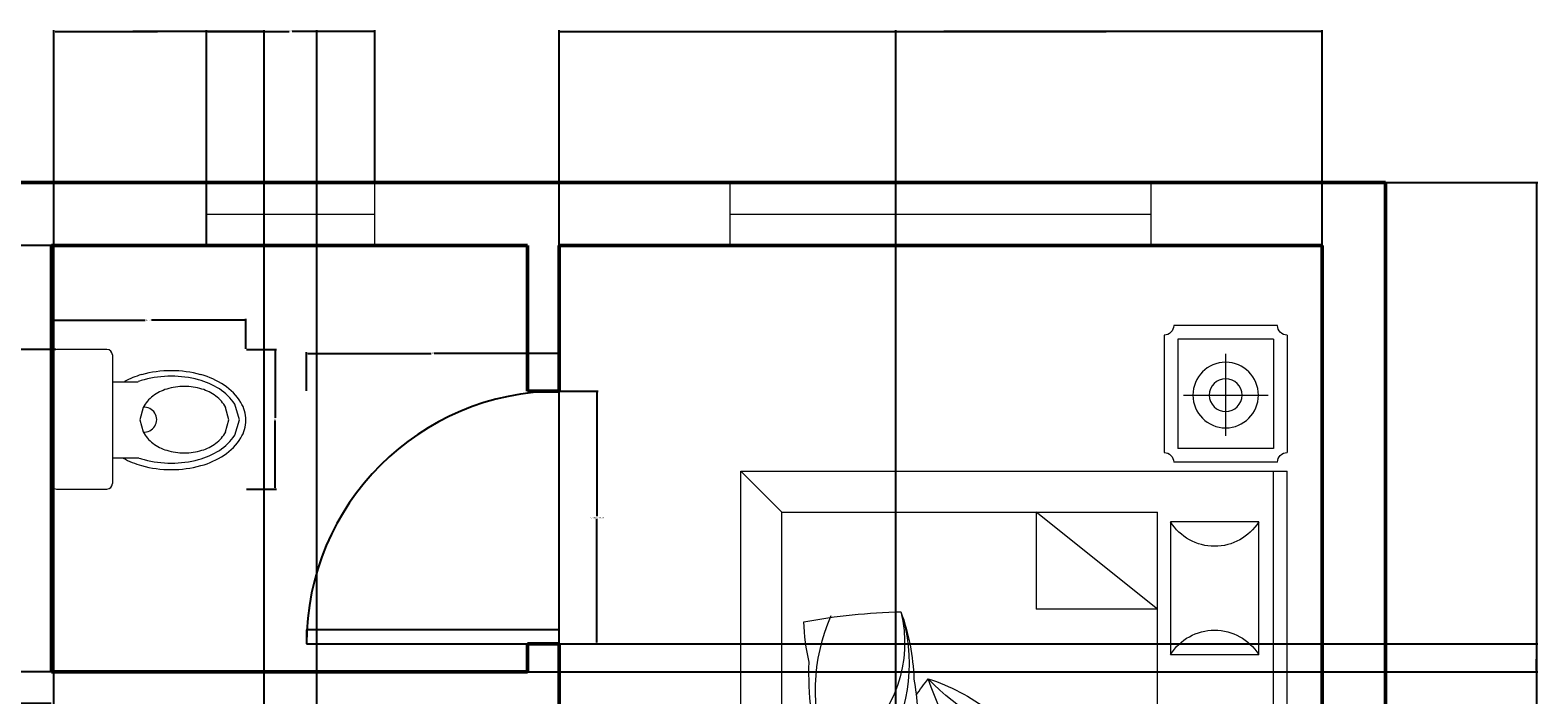
# Model space of a CAD drawing. Units: inches. Extents: x -108 to 1456, y -102 to 617.
# Tile 7 of 8: x 345 to 560, y 523 to 617. Entities that reach past the tile are written whole.
import ezdxf

# ---------------------------------------------------------------- set-up
doc = ezdxf.new("R2010")
doc.units = ezdxf.units.IN
for name, color, linetype, lineweight in [('A-ANNO-DIMS', 2, 'Continuous', 18), ('A-DOOR', 3, 'Continuous', 25), ('A-FLOR-FIXT', 9, 'Continuous', 20), ('A-FURN', 8, 'Continuous', 18), ('A-GLAZ', 4, 'Continuous', 18), ('A-WALL', 7, 'Continuous', 50)]:
    doc.layers.add(name, color=color, linetype=linetype, lineweight=lineweight)
doc.styles.get("Standard").update_dxf_attribs({"font": 'arial.ttf'})
doc.dimstyles.get("Standard").update_dxf_attribs({"dimtxt": 0.18, "dimasz": 0.18, "dimexe": 0.18, "dimexo": 0.0625, "dimgap": 0.09, "dimtad": 0, "dimtih": 1, "dimtoh": 1, "dimdec": 4, "dimzin": 0, "dimdsep": 46, "dimtxsty": 'Standard', "dimcen": 0.09, "dimadec": 0, "dimazin": 0, "dimtfac": 1, "dimtdec": 4, "dimtofl": 0, "dimtmove": 0, "dimatfit": 3, "dimfxl": 1, "dimtolj": 1, "dimtzin": 0, "dimarcsym": 0})

# ---------------------------------------------------------------- blocks, each defined once
blk = doc.blocks.new('A$C50B66110')
for p, q in [((0.0503, 1.9981), (0.4803, 1.9981)), ((0.1513, 1.6871), (0.1513, 1.9967)), ((0.5716, 1.9488), (0.5716, 2)), ((0.5716, 2), (2.0719, 2)), ((2.0719, 1.9488), (2.0719, 2)), ((2.5701, 1.9993), (2.1401, 1.9993)), ((0.0153, 1.9631), (0.0153, 1.5831)), ((0.0653, 1.9481), (0.0653, 1.5981)), ((0.0653, 1.9481), (0.4653, 1.9481)), ((0.4653, 1.9481), (0.4653, 1.5981)), ((0.5153, 1.9631), (0.5153, 1.5831)), ((2.0719, 1.9488), (0.5716, 1.9488)), ((0.5716, 1.9488), (0.5716, 0)), ((2.0719, 0), (2.0719, 1.9488)), ((2.1051, 1.9643), (2.1051, 1.5843)), ((2.1551, 1.9493), (2.1551, 1.5993)), ((2.5551, 1.9493), (2.1551, 1.9493)), ((2.5551, 1.9493), (2.5551, 1.5993)), ((2.6051, 1.9643), (2.6051, 1.5843)), ((0.7257, 1.5725), (0.7257, 1.8954)), ((0.7257, 1.8954), (1.2113, 1.8954)), ((1.2113, 1.8954), (1.2113, 1.5725)), ((1.4007, 1.5725), (1.4007, 1.8954)), ((1.4007, 1.8954), (1.8863, 1.8954)), ((1.8863, 1.8954), (1.8863, 1.5725)), ((2.3505, 1.62), (2.3505, 1.9295)), ((0, 1.8416), (0.2001, 1.8416)), ((2.5018, 1.7744), (2.2017, 1.7744)), ((0.0503, 1.5481), (0.4803, 1.5481)), ((0.0653, 1.5981), (0.4653, 1.5981)), ((1.2113, 1.5725), (0.7257, 1.5725)), ((1.8863, 1.5725), (1.4007, 1.5725)), ((2.5701, 1.5493), (2.1401, 1.5493)), ((2.5551, 1.5993), (2.1551, 1.5993)), ((1.5665, 1.5254), (1.5665, 1.0802)), ((1.5665, 1.5254), (1.9219, 1.0802)), ((1.9219, 1.0802), (1.5665, 1.0802)), ((0.5716, 0), (0.7216, 0.15)), ((2.0719, 0), (1.9219, 0.15)), ((0.5716, 0), (2.0719, 0))]:
    blk.add_line(p, q)
at = {"linetype": 'ByBlock'}
for p, q in [((0.2481, 1.9162), (0.2458, 1.9139)), ((0.2458, 1.9139), (0.2458, 1.7562)), ((0.2481, 1.9162), (0.4287, 1.9162)), ((0.2526, 1.9036), (0.2526, 1.8431)), ((0.3669, 1.9036), (0.2526, 1.9036)), ((0.3669, 1.8431), (0.3669, 1.9036)), ((0.3772, 1.9071), (0.3818, 1.9128)), ((0.3772, 1.7688), (0.3772, 1.9071)), ((0.3818, 1.9094), (0.3807, 1.9048)), ((0.3807, 1.9048), (0.3807, 1.8739)), ((0.3807, 1.9048), (0.3909, 1.8945)), ((0.3818, 1.9128), (0.4161, 1.9128)), ((0.3864, 1.9116), (0.3818, 1.9094)), ((0.3921, 1.8968), (0.3864, 1.9116)), ((0.3864, 1.9116), (0.4138, 1.9116)), ((0.3909, 1.8945), (0.3921, 1.8968)), ((0.3909, 1.8431), (0.3909, 1.8945)), ((0.4081, 1.8968), (0.3921, 1.8968)), ((0.4081, 1.8968), (0.4138, 1.9116)), ((0.4092, 1.8945), (0.4081, 1.8968)), ((0.4195, 1.9048), (0.4092, 1.8945)), ((0.4092, 1.8431), (0.4092, 1.8945)), ((0.4138, 1.9116), (0.4184, 1.9094)), ((0.4161, 1.9128), (0.4218, 1.9071)), ((0.4184, 1.9094), (0.4195, 1.9048)), ((0.4195, 1.9048), (0.4195, 1.8739)), ((0.4218, 1.9071), (0.4218, 1.7699)), ((0.4287, 1.9162), (0.4309, 1.9139)), ((0.4309, 1.9139), (0.4309, 1.7562)), ((0.2526, 1.8431), (0.3669, 1.8431)), ((0.2572, 1.8408), (0.2572, 1.8294)), ((0.3669, 1.8408), (0.2572, 1.8408)), ((0.2572, 1.8294), (0.3669, 1.8294)), ((0.2664, 1.8408), (0.2664, 1.8294)), ((0.2755, 1.8408), (0.2755, 1.8294)), ((0.2846, 1.8408), (0.2846, 1.8294)), ((0.2938, 1.8408), (0.2938, 1.8294)), ((0.3029, 1.8408), (0.3029, 1.8294)), ((0.3121, 1.8408), (0.3121, 1.8294)), ((0.3669, 1.8294), (0.3669, 1.8408)), ((0.3807, 1.8739), (0.3829, 1.8682)), ((0.3829, 1.8682), (0.3864, 1.8625)), ((0.3864, 1.8625), (0.3875, 1.8545)), ((0.3864, 1.8134), (0.3875, 1.8214)), ((0.3875, 1.8545), (0.3875, 1.8431)), ((0.3875, 1.8214), (0.3875, 1.8431)), ((0.3909, 1.8431), (0.3909, 1.7813)), ((0.4092, 1.8431), (0.4092, 1.7813)), ((0.4138, 1.8625), (0.4127, 1.8545)), ((0.4127, 1.8545), (0.4127, 1.8431)), ((0.4127, 1.8214), (0.4127, 1.8431)), ((0.4138, 1.8134), (0.4127, 1.8214)), ((0.4172, 1.8682), (0.4138, 1.8625)), ((0.4195, 1.8739), (0.4172, 1.8682)), ((0.3201, 1.8168), (0.2526, 1.8168)), ((0.2526, 1.8168), (0.2526, 1.7962)), ((0.2526, 1.7962), (0.3201, 1.7962)), ((0.2652, 1.7905), (0.2538, 1.7905)), ((0.2538, 1.7905), (0.2538, 1.7859)), ((0.2538, 1.7859), (0.2652, 1.7859)), ((0.2538, 1.7665), (0.2538, 1.7733)), ((0.2538, 1.7733), (0.2652, 1.7733)), ((0.2652, 1.7665), (0.2538, 1.7665)), ((0.2675, 1.8145), (0.2641, 1.8145)), ((0.2641, 1.8145), (0.2641, 1.8111)), ((0.2641, 1.8111), (0.2675, 1.8111)), ((0.2641, 1.8019), (0.2641, 1.7985)), ((0.2675, 1.8019), (0.2641, 1.8019)), ((0.2641, 1.7985), (0.2675, 1.7985)), ((0.2652, 1.7859), (0.2652, 1.7905)), ((0.2652, 1.7733), (0.2652, 1.7665)), ((0.2675, 1.8111), (0.2675, 1.8145)), ((0.2675, 1.7985), (0.2675, 1.8019)), ((0.2812, 1.7905), (0.2698, 1.7905)), ((0.2698, 1.7905), (0.2698, 1.7859)), ((0.2698, 1.7859), (0.2812, 1.7859)), ((0.2698, 1.7665), (0.2698, 1.7733)), ((0.2698, 1.7733), (0.2812, 1.7733)), ((0.2812, 1.7665), (0.2698, 1.7665)), ((0.2812, 1.7859), (0.2812, 1.7905)), ((0.2812, 1.7733), (0.2812, 1.7665)), ((0.2846, 1.8145), (0.2846, 1.8111)), ((0.2881, 1.8145), (0.2846, 1.8145)), ((0.2846, 1.8111), (0.2881, 1.8111)), ((0.2846, 1.8019), (0.2846, 1.7985)), ((0.2881, 1.8019), (0.2846, 1.8019)), ((0.2846, 1.7985), (0.2881, 1.7985)), ((0.2972, 1.7905), (0.2858, 1.7905)), ((0.2858, 1.7905), (0.2858, 1.7859)), ((0.2858, 1.7859), (0.2972, 1.7859)), ((0.2858, 1.7665), (0.2858, 1.7733)), ((0.2858, 1.7733), (0.2972, 1.7733)), ((0.2972, 1.7665), (0.2858, 1.7665)), ((0.2881, 1.8111), (0.2881, 1.8145)), ((0.2881, 1.7985), (0.2881, 1.8019)), ((0.2972, 1.7859), (0.2972, 1.7905)), ((0.2972, 1.7733), (0.2972, 1.7665)), ((0.3018, 1.7905), (0.3018, 1.7859)), ((0.3132, 1.7905), (0.3018, 1.7905)), ((0.3018, 1.7859), (0.3132, 1.7859)), ((0.3018, 1.7733), (0.3132, 1.7733)), ((0.3018, 1.7665), (0.3018, 1.7733)), ((0.3132, 1.7665), (0.3018, 1.7665)), ((0.3052, 1.8145), (0.3052, 1.8111)), ((0.3086, 1.8145), (0.3052, 1.8145)), ((0.3052, 1.8111), (0.3086, 1.8111)), ((0.3052, 1.8019), (0.3052, 1.7985)), ((0.3086, 1.8019), (0.3052, 1.8019)), ((0.3052, 1.7985), (0.3086, 1.7985)), ((0.3086, 1.8111), (0.3086, 1.8145)), ((0.3086, 1.7985), (0.3086, 1.8019)), ((0.3132, 1.7859), (0.3132, 1.7905)), ((0.3132, 1.7733), (0.3132, 1.7665)), ((0.3201, 1.7962), (0.3201, 1.8168)), ((0.3304, 1.8111), (0.3395, 1.8111)), ((0.3304, 1.8042), (0.3304, 1.8111)), ((0.3395, 1.8042), (0.3304, 1.8042)), ((0.3304, 1.7985), (0.3395, 1.7985)), ((0.3304, 1.7916), (0.3304, 1.7985)), ((0.3395, 1.7916), (0.3304, 1.7916)), ((0.3304, 1.7779), (0.3304, 1.7848)), ((0.3304, 1.7848), (0.3395, 1.7848)), ((0.3395, 1.7779), (0.3304, 1.7779)), ((0.3304, 1.7722), (0.3395, 1.7722)), ((0.3304, 1.7653), (0.3304, 1.7722)), ((0.3395, 1.8111), (0.3395, 1.8042)), ((0.3395, 1.7985), (0.3395, 1.7916)), ((0.3395, 1.7848), (0.3395, 1.7779)), ((0.3395, 1.7722), (0.3395, 1.7653)), ((0.3441, 1.8042), (0.3441, 1.8111)), ((0.3441, 1.8111), (0.3532, 1.8111)), ((0.3532, 1.8042), (0.3441, 1.8042)), ((0.3441, 1.7985), (0.3532, 1.7985)), ((0.3441, 1.7916), (0.3441, 1.7985)), ((0.3532, 1.7916), (0.3441, 1.7916)), ((0.3441, 1.7779), (0.3441, 1.7848)), ((0.3441, 1.7848), (0.3532, 1.7848)), ((0.3532, 1.7779), (0.3441, 1.7779)), ((0.3441, 1.7722), (0.3532, 1.7722)), ((0.3441, 1.7653), (0.3441, 1.7722)), ((0.3532, 1.8111), (0.3532, 1.8042)), ((0.3532, 1.7985), (0.3532, 1.7916)), ((0.3532, 1.7848), (0.3532, 1.7779)), ((0.3532, 1.7722), (0.3532, 1.7653)), ((0.3578, 1.8111), (0.3669, 1.8111)), ((0.3578, 1.8042), (0.3578, 1.8111)), ((0.3669, 1.8042), (0.3578, 1.8042)), ((0.3578, 1.7985), (0.3669, 1.7985)), ((0.3578, 1.7916), (0.3578, 1.7985)), ((0.3669, 1.7916), (0.3578, 1.7916)), ((0.3578, 1.7791), (0.3578, 1.7859)), ((0.3578, 1.7859), (0.3669, 1.7859)), ((0.3669, 1.7791), (0.3578, 1.7791)), ((0.3578, 1.7653), (0.3578, 1.7722)), ((0.3578, 1.7722), (0.3669, 1.7722)), ((0.3669, 1.8111), (0.3669, 1.8042)), ((0.3669, 1.7985), (0.3669, 1.7916)), ((0.3669, 1.7859), (0.3669, 1.7791)), ((0.3669, 1.7722), (0.3669, 1.7653)), ((0.3829, 1.7631), (0.3772, 1.7688)), ((0.3807, 1.8019), (0.3829, 1.8076)), ((0.3807, 1.7711), (0.3807, 1.8019)), ((0.3807, 1.7711), (0.3909, 1.7813)), ((0.3818, 1.7665), (0.3807, 1.7711)), ((0.3864, 1.7642), (0.3818, 1.7665)), ((0.3829, 1.8076), (0.3864, 1.8134)), ((0.3921, 1.7791), (0.3864, 1.7642)), ((0.3909, 1.7813), (0.3921, 1.7791)), ((0.4081, 1.7791), (0.3921, 1.7791)), ((0.4024, 1.7676), (0.3989, 1.7676)), ((0.3989, 1.7676), (0.3991, 1.7578)), ((0.403, 1.7585), (0.4024, 1.7676)), ((0.4092, 1.7813), (0.4081, 1.7791)), ((0.4081, 1.7791), (0.4138, 1.7642)), ((0.4195, 1.7711), (0.4092, 1.7813)), ((0.4172, 1.8076), (0.4138, 1.8134)), ((0.4138, 1.7642), (0.4184, 1.7665)), ((0.4218, 1.7699), (0.4161, 1.7631)), ((0.4195, 1.8019), (0.4172, 1.8076)), ((0.4184, 1.7665), (0.4195, 1.7711)), ((0.4195, 1.7711), (0.4195, 1.8019)), ((0.4378, 1.7742), (0.4309, 1.7768)), ((0.4309, 1.7722), (0.436, 1.7708)), ((0.436, 1.7708), (0.4406, 1.7672)), ((0.441, 1.771), (0.4378, 1.7742)), ((0.4406, 1.7672), (0.4418, 1.7656)), ((0.4434, 1.7688), (0.441, 1.771)), ((0.4477, 1.7704), (0.4434, 1.7688)), ((0.4497, 1.7684), (0.4477, 1.7704)), ((0.4481, 1.765), (0.4497, 1.7684)), ((0.4509, 1.7672), (0.4481, 1.765)), ((0.4539, 1.764), (0.4509, 1.7672)), ((0.2458, 1.7562), (0.2481, 1.7539)), ((0.4, 1.7539), (0.2481, 1.7539)), ((0.3395, 1.7653), (0.3304, 1.7653)), ((0.3532, 1.7653), (0.3441, 1.7653)), ((0.3669, 1.7653), (0.3578, 1.7653)), ((0.399, 1.7631), (0.3829, 1.7631)), ((0.3864, 1.7642), (0.399, 1.7642)), ((0.3991, 1.7578), (0.4019, 1.7462)), ((0.4019, 1.7462), (0.4047, 1.7353)), ((0.4026, 1.7254), (0.4021, 1.7198)), ((0.4021, 1.7198), (0.4088, 1.7187)), ((0.4088, 1.7187), (0.4023, 1.7147)), ((0.4023, 1.7147), (0.4028, 1.7085)), ((0.4026, 1.7642), (0.4138, 1.7642)), ((0.4051, 1.7279), (0.4026, 1.7254)), ((0.4161, 1.7631), (0.4027, 1.7631)), ((0.4047, 1.7511), (0.403, 1.7585)), ((0.4287, 1.7539), (0.404, 1.7539)), ((0.4047, 1.7353), (0.4044, 1.7293)), ((0.4044, 1.7293), (0.4051, 1.7279)), ((0.4074, 1.7402), (0.4047, 1.7511)), ((0.4081, 1.7346), (0.4074, 1.7402)), ((0.4079, 1.7286), (0.4081, 1.7346)), ((0.4121, 1.7256), (0.4079, 1.7286)), ((0.4111, 1.7203), (0.4121, 1.7256)), ((0.4123, 1.7057), (0.4111, 1.7203)), ((0.4309, 1.7562), (0.4287, 1.7539)), ((0.4443, 1.7658), (0.4418, 1.7633)), ((0.4418, 1.7656), (0.4443, 1.7658)), ((0.4418, 1.7633), (0.4511, 1.7551)), ((0.4511, 1.7551), (0.4662, 1.7422)), ((0.4515, 1.7573), (0.4539, 1.764)), ((0.4577, 1.7605), (0.4515, 1.7573)), ((0.463, 1.7555), (0.4577, 1.7605)), ((0.4618, 1.7482), (0.463, 1.7555)), ((0.467, 1.7515), (0.4618, 1.7482)), ((0.4664, 1.7418), (0.4741, 1.72)), ((0.4714, 1.7468), (0.467, 1.7515)), ((0.4696, 1.7418), (0.4714, 1.7468)), ((0.4766, 1.7425), (0.4697, 1.7418)), ((0.4741, 1.72), (0.4708, 1.7027)), ((0.472, 1.733), (0.4787, 1.7356)), ((0.4794, 1.7332), (0.472, 1.733)), ((0.4761, 1.7233), (0.481, 1.7279)), ((0.4824, 1.7233), (0.4761, 1.7233)), ((0.4764, 1.7154), (0.4835, 1.7175)), ((0.4824, 1.7119), (0.4764, 1.7154)), ((0.4787, 1.7356), (0.4766, 1.7425)), ((0.481, 1.7279), (0.4794, 1.7332)), ((0.4815, 1.7073), (0.4824, 1.7119)), ((0.4835, 1.7175), (0.4824, 1.7233)), ((0.4028, 1.7085), (0.4102, 1.7078)), ((0.4102, 1.7078), (0.4037, 1.7027)), ((0.4037, 1.7027), (0.4067, 1.6974)), ((0.4067, 1.6974), (0.4137, 1.6988)), ((0.4137, 1.6988), (0.4104, 1.6923)), ((0.4104, 1.6923), (0.4139, 1.6881)), ((0.4211, 1.6946), (0.4123, 1.7057)), ((0.4139, 1.6881), (0.4192, 1.692)), ((0.4192, 1.692), (0.4183, 1.6858)), ((0.4183, 1.6858), (0.4227, 1.683)), ((0.4333, 1.6881), (0.4211, 1.6946)), ((0.4227, 1.683), (0.4283, 1.6876)), ((0.4283, 1.6876), (0.4276, 1.68)), ((0.4276, 1.68), (0.4324, 1.6786)), ((0.4324, 1.6786), (0.4354, 1.6849)), ((0.4472, 1.6869), (0.4333, 1.6881)), ((0.4354, 1.6849), (0.4382, 1.6786)), ((0.4382, 1.6786), (0.4421, 1.6782)), ((0.4421, 1.6782), (0.4437, 1.6849)), ((0.4437, 1.6849), (0.4463, 1.6775)), ((0.4463, 1.6775), (0.4507, 1.6786)), ((0.4606, 1.6927), (0.4472, 1.6869)), ((0.4507, 1.6786), (0.4509, 1.6849)), ((0.4509, 1.6849), (0.4562, 1.6802)), ((0.4562, 1.6802), (0.4599, 1.6821)), ((0.4592, 1.689), (0.4641, 1.683)), ((0.4599, 1.6821), (0.4592, 1.689)), ((0.4708, 1.7027), (0.4606, 1.6927)), ((0.4641, 1.683), (0.4678, 1.6863)), ((0.465, 1.6925), (0.4715, 1.6897)), ((0.4678, 1.6863), (0.465, 1.6925)), ((0.4745, 1.6925), (0.4713, 1.6988)), ((0.4713, 1.6988), (0.478, 1.6967)), ((0.4715, 1.6897), (0.4745, 1.6925)), ((0.4743, 1.7075), (0.4815, 1.7073)), ((0.4798, 1.7013), (0.4743, 1.7075)), ((0.478, 1.6967), (0.4798, 1.7013)), ((0.7216, 1.5254), (1.9219, 1.5254)), ((0.7216, 1.5254), (0.7216, 0.15)), ((1.9219, 0.15), (1.9219, 1.5254)), ((0.7216, 0.15), (1.9219, 0.15))]:
    blk.add_line(p, q, dxfattribs=at)
for centre, radius in [((0.1513, 1.8416), 0.12), ((0.1513, 1.8416), 0.06), ((2.3505, 1.7744), 0.12), ((2.3505, 1.7744), 0.06)]:
    blk.add_circle(centre, radius)
for centre, radius, start, end in [((0.0153, 1.9981), 0.035, 270, 0), ((0.5153, 1.9981), 0.035, 180, 270), ((2.1051, 1.9993), 0.035, 270, 0), ((2.6051, 1.9993), 0.035, 180, 270), ((0.6244, 1.734), 0.1906, 302.1202, 57.8798), ((1.3126, 1.734), 0.1906, 122.1202, 237.8798), ((1.2994, 1.734), 0.1906, 302.1202, 57.8798), ((1.9876, 1.734), 0.1906, 122.1202, 237.8798), ((0.0153, 1.5481), 0.035, 0, 90), ((0.5153, 1.5481), 0.035, 90, 180), ((2.1051, 1.5493), 0.035, 0, 90), ((2.6051, 1.5493), 0.035, 90, 180), ((1.1502, 0.7366), 0.3575, 102.4782, 140.4625), ((0.328, 0.4368), 0.9879, 28.4971, 41.0566), ((1.9117, 1.3157), 0.8697, 195.336, 226.4193), ((0.9996, 0.4307), 0.548, 103.2034, 117.0362), ((1.656, 1.7093), 1.0798, 223.6306, 251.4288), ((0.4482, 0.4408), 0.5655, 5.3391, 57.6895), ((1.8226, 1.3753), 1.1652, 203.0642, 220.3209), ((0.4548, 0.5307), 0.4879, 10.6986, 52.6864), ((0.5648, 0.4378), 0.7874, 18.3527, 36.6851), ((-0.0179, 2.4352), 2.1977, 305.2966, 307.2418), ((1.5981, 0.9345), 0.734, 205.259, 216.9351), ((1.4166, 0.4903), 0.3575, 154.0418, 192.0262), ((1.3672, 0.0075), 0.6085, 71.81, 120.1351), ((1.1403, -0.3401), 0.9879, 80.0607, 92.6202), ((1.2867, -0.154), 0.7874, 69.9163, 88.2487), ((1.4431, 0.1219), 0.4774, 76.1849, 142.0017), ((-0.6401, 0.6314), 2.1977, 349.4884, 358.8054), ((-0.0179, 2.4352), 2.1977, 297.9248, 299.3793), ((1.5626, 0.1822), 0.548, 154.767, 168.5998), ((1.3343, 1.4141), 1.1652, 254.6278, 271.8845), ((1.2678, 0.9611), 0.6885, 250.2936, 293.6414), ((1.5399, 0.9642), 0.734, 256.8226, 268.4988)]:
    blk.add_arc(centre, radius, start, end)
blk = doc.blocks.new('A$C44022395')
for p, q in [((0, 0.6877), (0, 0.5044)), ((0.4866, 0.7077), (0.02, 0.7077)), ((0.5066, 0.5044), (0.5066, 0.6877)), ((0.4866, 0.4844), (0.02, 0.4844)), ((0.1134, 0.4844), (0.1134, 0.389)), ((0.3892, 0.4844), (0.3892, 0.3908)), ((0.2517, 0.3846), (0.2074, 0.3731)), ((0.2959, 0.3731), (0.2517, 0.3846)), ((0.2074, 0.0734), (0.2517, 0.0619)), ((0.2517, 0.0619), (0.2959, 0.0734)), ((0.1955, 0.0404), (0.2517, 0.0238)), ((0.2517, 0.0238), (0.3078, 0.0404))]:
    blk.add_line(p, q)
for centre, radius, start, end in [((0.02, 0.6877), 0.02, 90, 180), ((0.4866, 0.6877), 0.02, 0, 90), ((0.02, 0.5044), 0.02, 180, 270), ((0.4866, 0.5044), 0.02, 270, 0), ((0.3656, 0.3016), 0.291, 150.4483, 164.652), ((0.1344, 0.3016), 0.291, 15.348, 28.5058), ((0.3673, 0.3006), 0.2695, 161.3359, 165.1916), ((0.136, 0.3006), 0.2695, 14.8084, 19.6606), ((0.4778, 0.2708), 0.4073, 164.652, 180), ((0.4797, 0.2708), 0.3857, 165.1916, 180), ((0.2995, 0.2376), 0.1665, 143.1832, 162.7734), ((0.2702, 0.2595), 0.1299, 118.958, 143.1832), ((0.2518, 0.3688), 0.0451, 174.4043, 5.5957), ((0.2331, 0.2595), 0.1299, 36.8168, 61.042), ((0.2038, 0.2376), 0.1665, 17.2266, 36.8168), ((0.0236, 0.2708), 0.3857, 0, 14.8084), ((0.0221, 0.2708), 0.4073, 0, 15.348), ((0.3457, 0.2233), 0.2148, 162.7734, 180), ((0.1576, 0.2233), 0.2148, 0, 17.2266), ((0.4778, 0.2708), 0.4073, 180, 195.348), ((0.4797, 0.2708), 0.3857, 180, 194.8084), ((0.3457, 0.2233), 0.2148, 180, 197.2266), ((0.1576, 0.2233), 0.2148, 342.7734, 0), ((0.0236, 0.2708), 0.3857, 345.1916, 0), ((0.0221, 0.2708), 0.4073, 344.652, 0), ((0.3673, 0.2411), 0.2695, 194.8084, 212.5477), ((0.136, 0.2411), 0.2695, 327.4523, 345.1916), ((0.3656, 0.24), 0.291, 195.348, 213.5296), ((0.2995, 0.2089), 0.1665, 197.2266, 216.8168), ((0.2038, 0.2089), 0.1665, 323.1832, 342.7734), ((0.1344, 0.24), 0.291, 326.4704, 344.652), ((0.2947, 0.193), 0.2059, 213.5296, 237.9903), ((0.2963, 0.1958), 0.1852, 212.5477, 237.0167), ((0.2702, 0.187), 0.1299, 216.8168, 241.042), ((0.2331, 0.187), 0.1299, 298.958, 323.1832), ((0.207, 0.1958), 0.1852, 302.9833, 327.4523), ((0.2053, 0.193), 0.2059, 302.0097, 326.4704), ((0.25, 0.1215), 0.1215, 237.9903, 270), ((0.25, 0.1215), 0.1215, 270, 302.0097)]:
    blk.add_arc(centre, radius, start, end)
blk = doc.blocks.new('DOOR-36-SWING-WITH-CLOSURE')
for p, q in [((36, 36), (0, 36)), ((36, 36), (34, 36)), ((34, 36), (34, 0)), ((36, 0), (36, 36)), ((34, 0), (36, 0))]:
    blk.add_line(p, q)
blk.add_arc((36, 36), 36, 180, 270)
blk = doc.blocks.new('WIN-60-WALL-9')
for p, q in [((0, 0), (0, 9)), ((60, 0), (60, 9)), ((0, 4.5), (60, 4.5))]:
    blk.add_line(p, q)
blk = doc.blocks.new('*D14')
at = {"layer": 'A-ANNO-DIMS', "color": 0, "lineweight": -2, "transparency": 16777216}
for p, q in [((420.66, 566.02), (426.17, 566.02)), ((425.99, 565.84), (425.99, 548.21)), ((425.99, 530.2), (425.99, 547.84)), ((420.66, 530.02), (426.17, 530.02))]:
    blk.add_line(p, q, dxfattribs=at)
at = {"layer": 'A-ANNO-DIMS', "color": 0, "transparency": 16777216}
for points in [[(425.96, 565.84), (426.02, 565.84), (425.99, 566.02)], [(425.96, 530.2), (426.02, 530.2), (425.99, 530.02)]]:
    blk.add_solid(points, dxfattribs=at)
at = {"layer": 'Defpoints', "color": 0, "transparency": 16777216}
for p in [(420.59, 566.02), (420.59, 530.02), (425.99, 530.02)]:
    blk.add_point(p, dxfattribs=at)
at = {"layer": 'A-ANNO-DIMS', "color": 0, "transparency": 16777216, "insert": (425.99, 548.02), "char_height": 0.18, "attachment_point": 5}
blk.add_mtext('\\A1;CLOSER DOOR 36', dxfattribs=at)
blk = doc.blocks.new('*D15')
at = {"layer": 'A-ANNO-DIMS', "color": 0, "lineweight": -2, "transparency": 16777216}
for p, q in [((384.59, 566.09), (384.59, 571.6)), ((420.59, 566.09), (420.59, 571.6)), ((384.77, 571.42), (402.38, 571.42)), ((420.41, 571.42), (402.81, 571.42))]:
    blk.add_line(p, q, dxfattribs=at)
at = {"layer": 'A-ANNO-DIMS', "color": 0, "transparency": 16777216}
for points in [[(384.77, 571.45), (384.77, 571.39), (384.59, 571.42)], [(420.41, 571.45), (420.41, 571.39), (420.59, 571.42)]]:
    blk.add_solid(points, dxfattribs=at)
at = {"layer": 'Defpoints', "color": 0, "transparency": 16777216}
for p in [(420.59, 571.42), (384.59, 566.02), (420.59, 566.02)]:
    blk.add_point(p, dxfattribs=at)
at = {"layer": 'A-ANNO-DIMS', "color": 0, "transparency": 16777216, "insert": (402.59, 571.42), "char_height": 0.18, "attachment_point": 5}
blk.add_mtext('\\A1;36', dxfattribs=at)
blk = doc.blocks.new('*D24')
at = {"layer": 'A-ANNO-DIMS', "color": 0, "lineweight": -2, "transparency": 16777216}
for p, q in [((348.17, 572.05), (348.17, 576.33)), ((348.35, 576.15), (361.6, 576.15)), ((375.78, 576.15), (362.53, 576.15)), ((375.96, 572.05), (375.96, 576.33))]:
    blk.add_line(p, q, dxfattribs=at)
at = {"layer": 'A-ANNO-DIMS', "color": 0, "transparency": 16777216}
for points in [[(348.35, 576.18), (348.35, 576.12), (348.17, 576.15)], [(375.78, 576.18), (375.78, 576.12), (375.96, 576.15)]]:
    blk.add_solid(points, dxfattribs=at)
at = {"layer": 'Defpoints', "color": 0, "transparency": 16777216}
for p in [(348.17, 576.15), (348.17, 571.98), (375.96, 571.98)]:
    blk.add_point(p, dxfattribs=at)
at = {"layer": 'A-ANNO-DIMS', "color": 0, "transparency": 16777216, "insert": (362.07, 576.15), "char_height": 0.18, "attachment_point": 5}
blk.add_mtext('\\A1;WC 28', dxfattribs=at)
blk = doc.blocks.new('*D25')
at = {"layer": 'A-ANNO-DIMS', "color": 0, "lineweight": -2, "transparency": 16777216}
for p, q in [((376.03, 571.98), (380.31, 571.98)), ((380.13, 571.8), (380.13, 562.22)), ((380.13, 552.26), (380.13, 561.85)), ((376.03, 552.08), (380.31, 552.08))]:
    blk.add_line(p, q, dxfattribs=at)
at = {"layer": 'A-ANNO-DIMS', "color": 0, "transparency": 16777216}
for points in [[(380.1, 571.8), (380.16, 571.8), (380.13, 571.98)], [(380.1, 552.26), (380.16, 552.26), (380.13, 552.08)]]:
    blk.add_solid(points, dxfattribs=at)
at = {"layer": 'Defpoints', "color": 0, "transparency": 16777216}
for p in [(375.96, 571.98), (380.13, 571.98), (375.96, 552.08)]:
    blk.add_point(p, dxfattribs=at)
at = {"layer": 'A-ANNO-DIMS', "color": 0, "transparency": 16777216, "insert": (380.13, 562.03), "char_height": 0.18, "attachment_point": 5}
blk.add_mtext('\\A1;20', dxfattribs=at)
blk = doc.blocks.new('*D35')
at = {"layer": 'A-ANNO-DIMS', "color": 0, "lineweight": -2, "transparency": 16777216}
for p, q in [((538.41, 595.77), (560.05, 595.77)), ((559.87, 595.59), (559.87, 385.96)), ((559.87, 175.95), (559.87, 385.59)), ((538.41, 175.77), (560.05, 175.77))]:
    blk.add_line(p, q, dxfattribs=at)
at = {"layer": 'A-ANNO-DIMS', "color": 0, "transparency": 16777216}
for points in [[(559.84, 595.59), (559.9, 595.59), (559.87, 595.77)], [(559.84, 175.95), (559.9, 175.95), (559.87, 175.77)]]:
    blk.add_solid(points, dxfattribs=at)
at = {"layer": 'Defpoints', "color": 0, "transparency": 16777216}
for p in [(538.34, 595.77), (559.87, 595.77), (538.34, 175.77)]:
    blk.add_point(p, dxfattribs=at)
at = {"layer": 'A-ANNO-DIMS', "color": 0, "transparency": 16777216, "insert": (559.87, 385.77), "char_height": 0.18, "attachment_point": 5}
blk.add_mtext('\\A1;420', dxfattribs=at)
blk = doc.blocks.new('*D38')
at = {"layer": 'A-ANNO-DIMS', "color": 0, "lineweight": -2, "transparency": 16777216}
for p, q in [((420.59, 586.84), (420.59, 617.48)), ((420.77, 617.3), (474.51, 617.3)), ((529.16, 617.3), (475.43, 617.3)), ((529.34, 586.84), (529.34, 617.48))]:
    blk.add_line(p, q, dxfattribs=at)
at = {"layer": 'A-ANNO-DIMS', "color": 0, "transparency": 16777216}
for points in [[(420.77, 617.33), (420.77, 617.27), (420.59, 617.3)], [(529.16, 617.33), (529.16, 617.27), (529.34, 617.3)]]:
    blk.add_solid(points, dxfattribs=at)
at = {"layer": 'Defpoints', "color": 0, "transparency": 16777216}
for p in [(529.34, 617.3), (420.59, 586.77), (529.34, 586.77)]:
    blk.add_point(p, dxfattribs=at)
at = {"layer": 'A-ANNO-DIMS', "color": 0, "transparency": 16777216, "insert": (474.97, 617.3), "char_height": 0.18, "attachment_point": 5}
blk.add_mtext('\\A1;108.75', dxfattribs=at)
blk = doc.blocks.new('*D46')
at = {"layer": 'A-ANNO-DIMS', "color": 0, "lineweight": -2, "transparency": 16777216}
for p, q in [((348.2, 526.02), (204.64, 526.02)), ((204.82, 525.84), (204.82, 523.96)), ((204.82, 521.7), (204.82, 523.59)), ((348.2, 521.52), (204.64, 521.52))]:
    blk.add_line(p, q, dxfattribs=at)
at = {"layer": 'A-ANNO-DIMS', "color": 0, "transparency": 16777216}
for points in [[(204.79, 525.84), (204.85, 525.84), (204.82, 526.02)], [(204.79, 521.7), (204.85, 521.7), (204.82, 521.52)]]:
    blk.add_solid(points, dxfattribs=at)
at = {"layer": 'Defpoints', "color": 0, "transparency": 16777216}
for p in [(348.27, 526.02), (204.82, 521.52), (348.27, 521.52)]:
    blk.add_point(p, dxfattribs=at)
at = {"layer": 'A-ANNO-DIMS', "color": 0, "transparency": 16777216, "insert": (204.82, 523.77), "char_height": 0.18, "attachment_point": 5}
blk.add_mtext('\\A1;4.5', dxfattribs=at)
blk = doc.blocks.new('*D47')
at = {"layer": 'A-ANNO-DIMS', "color": 0, "lineweight": -2, "transparency": 16777216}
for p, q in [((348.59, 586.84), (348.59, 617.48)), ((348.77, 617.3), (359.07, 617.3)), ((370.16, 617.3), (359.87, 617.3)), ((370.34, 586.84), (370.34, 617.48))]:
    blk.add_line(p, q, dxfattribs=at)
at = {"layer": 'A-ANNO-DIMS', "color": 0, "transparency": 16777216}
for points in [[(348.77, 617.33), (348.77, 617.27), (348.59, 617.3)], [(370.16, 617.33), (370.16, 617.27), (370.34, 617.3)]]:
    blk.add_solid(points, dxfattribs=at)
at = {"layer": 'Defpoints', "color": 0, "transparency": 16777216}
for p in [(370.34, 617.3), (348.59, 586.77), (370.34, 586.77)]:
    blk.add_point(p, dxfattribs=at)
at = {"layer": 'A-ANNO-DIMS', "color": 0, "transparency": 16777216, "insert": (359.47, 617.3), "char_height": 0.18, "attachment_point": 5}
blk.add_mtext('\\A1;21.75', dxfattribs=at)
blk = doc.blocks.new('*D48')
at = {"layer": 'A-ANNO-DIMS', "color": 0, "lineweight": -2, "transparency": 16777216}
for p, q in [((370.34, 595.84), (370.34, 617.48)), ((370.52, 617.3), (382.12, 617.3)), ((394.16, 617.3), (382.56, 617.3)), ((394.34, 595.84), (394.34, 617.48))]:
    blk.add_line(p, q, dxfattribs=at)
at = {"layer": 'A-ANNO-DIMS', "color": 0, "transparency": 16777216}
for points in [[(370.52, 617.33), (370.52, 617.27), (370.34, 617.3)], [(394.16, 617.33), (394.16, 617.27), (394.34, 617.3)]]:
    blk.add_solid(points, dxfattribs=at)
at = {"layer": 'Defpoints', "color": 0, "transparency": 16777216}
for p in [(394.34, 617.3), (370.34, 595.77), (394.34, 595.77)]:
    blk.add_point(p, dxfattribs=at)
at = {"layer": 'A-ANNO-DIMS', "color": 0, "transparency": 16777216, "insert": (382.34, 617.3), "char_height": 0.18, "attachment_point": 5}
blk.add_mtext('\\A1;24', dxfattribs=at)
blk = doc.blocks.new('*D50')
at = {"layer": 'A-ANNO-DIMS', "color": 0, "lineweight": -2, "transparency": 16777216}
for p, q in [((416.156823, 530.024278), (560.049323, 530.024278)), ((559.869323, 529.844278), (559.869323, 528.204278)), ((559.869323, 526.204278), (559.869323, 527.844278)), ((416.156823, 526.024278), (560.049323, 526.024278))]:
    blk.add_line(p, q, dxfattribs=at)
at = {"layer": 'A-ANNO-DIMS', "color": 0, "transparency": 16777216}
for points in [[(559.839323, 529.844278), (559.899323, 529.844278), (559.869323, 530.024278)], [(559.839323, 526.204278), (559.899323, 526.204278), (559.869323, 526.024278)]]:
    blk.add_solid(points, dxfattribs=at)
at = {"layer": 'Defpoints', "color": 0, "transparency": 16777216}
for p in [(416.094323, 530.024278), (559.869323, 530.024278), (416.094323, 526.024278)]:
    blk.add_point(p, dxfattribs=at)
at = {"layer": 'A-ANNO-DIMS', "color": 0, "transparency": 16777216, "insert": (559.869323, 528.024278), "char_height": 0.18, "attachment_point": 5}
blk.add_mtext('\\A1;4', dxfattribs=at)
blk = doc.blocks.new('*D51')
at = {"layer": 'A-ANNO-DIMS', "color": 0, "lineweight": -2, "transparency": 16777216}
for p, q in [((348.53, 586.77), (204.64, 586.77)), ((204.82, 586.59), (204.82, 579.56)), ((204.82, 572.16), (204.82, 579.2)), ((348.89, 571.98), (204.64, 571.98))]:
    blk.add_line(p, q, dxfattribs=at)
at = {"layer": 'A-ANNO-DIMS', "color": 0, "transparency": 16777216}
for points in [[(204.79, 586.59), (204.85, 586.59), (204.82, 586.77)], [(204.79, 572.16), (204.85, 572.16), (204.82, 571.98)]]:
    blk.add_solid(points, dxfattribs=at)
at = {"layer": 'Defpoints', "color": 0, "transparency": 16777216}
for p in [(348.59, 586.77), (204.82, 571.98), (348.95, 571.98)]:
    blk.add_point(p, dxfattribs=at)
at = {"layer": 'A-ANNO-DIMS', "color": 0, "transparency": 16777216, "insert": (204.82, 579.38), "char_height": 0.18, "attachment_point": 5}
blk.add_mtext('\\A1;14.79', dxfattribs=at)
blk = doc.blocks.new('*D57')
at = {"layer": 'A-ANNO-DIMS', "color": 0, "lineweight": -2, "transparency": 16777216}
for p, q in [((468.59, 449.59), (468.59, 617.48)), ((468.77, 617.3), (498.57, 617.3)), ((529.16, 617.3), (499.36, 617.3)), ((529.34, 449.59), (529.34, 617.48))]:
    blk.add_line(p, q, dxfattribs=at)
at = {"layer": 'A-ANNO-DIMS', "color": 0, "transparency": 16777216}
for points in [[(468.77, 617.33), (468.77, 617.27), (468.59, 617.3)], [(529.16, 617.33), (529.16, 617.27), (529.34, 617.3)]]:
    blk.add_solid(points, dxfattribs=at)
at = {"layer": 'Defpoints', "color": 0, "transparency": 16777216}
for p in [(529.34, 617.3), (468.59, 449.52), (529.34, 449.52)]:
    blk.add_point(p, dxfattribs=at)
at = {"layer": 'A-ANNO-DIMS', "color": 0, "transparency": 16777216, "insert": (498.97, 617.3), "char_height": 0.18, "attachment_point": 5}
blk.add_mtext('\\A1;60.75', dxfattribs=at)
blk = doc.blocks.new('*D62')
at = {"layer": 'A-ANNO-DIMS', "color": 0, "lineweight": -2, "transparency": 16777216}
for p, q in [((348.59, 314.09), (348.59, 617.48)), ((348.77, 617.3), (363.38, 617.3)), ((378.41, 617.3), (363.81, 617.3)), ((378.59, 314.09), (378.59, 617.48))]:
    blk.add_line(p, q, dxfattribs=at)
at = {"layer": 'A-ANNO-DIMS', "color": 0, "transparency": 16777216}
for points in [[(348.77, 617.33), (348.77, 617.27), (348.59, 617.3)], [(378.41, 617.33), (378.41, 617.27), (378.59, 617.3)]]:
    blk.add_solid(points, dxfattribs=at)
at = {"layer": 'Defpoints', "color": 0, "transparency": 16777216}
for p in [(378.59, 617.3), (348.59, 314.02), (378.59, 314.02)]:
    blk.add_point(p, dxfattribs=at)
at = {"layer": 'A-ANNO-DIMS', "color": 0, "transparency": 16777216, "insert": (363.59, 617.3), "char_height": 0.18, "attachment_point": 5}
blk.add_mtext('\\A1;30', dxfattribs=at)
blk = doc.blocks.new('*D63')
at = {"layer": 'A-ANNO-DIMS', "color": 0, "lineweight": -2, "transparency": 16777216}
for p, q in [((378.59, 314.09), (378.59, 617.48)), ((378.77, 617.3), (382.09, 617.3)), ((385.91, 617.3), (382.6, 617.3)), ((386.09, 314.09), (386.09, 617.48))]:
    blk.add_line(p, q, dxfattribs=at)
at = {"layer": 'A-ANNO-DIMS', "color": 0, "transparency": 16777216}
for points in [[(378.77, 617.33), (378.77, 617.27), (378.59, 617.3)], [(385.91, 617.33), (385.91, 617.27), (386.09, 617.3)]]:
    blk.add_solid(points, dxfattribs=at)
at = {"layer": 'Defpoints', "color": 0, "transparency": 16777216}
for p in [(386.09, 617.3), (378.59, 314.02), (386.09, 314.02)]:
    blk.add_point(p, dxfattribs=at)
at = {"layer": 'A-ANNO-DIMS', "color": 0, "transparency": 16777216, "insert": (382.34, 617.3), "char_height": 0.18, "attachment_point": 5}
blk.add_mtext('\\A1;7.5', dxfattribs=at)

msp = doc.modelspace()

# ---------------------------------------------------------------- linework, layer by layer
at = {"layer": 'A-DOOR'}
for p, q in [((418.5943, 565.9687), (418.5943, 566.0243)), ((418.5943, 566.0243), (420.5943, 566.0243)), ((420.5943, 530.0243), (416.0943, 530.0243)), ((420.5943, 530.0243), (418.5943, 530.0243))]:
    msp.add_line(p, q, dxfattribs=at)
msp.add_arc((420.5943, 530.0243), 36, 90, 93.184739, dxfattribs=at)
at = {"layer": 'A-GLAZ'}
for p, q in [((370.3443, 586.7743), (370.3443, 595.7743)), ((394.3443, 586.7743), (394.3443, 595.7743)), ((370.3443, 591.2743), (394.3443, 591.2743))]:
    msp.add_line(p, q, dxfattribs=at)
at = {"layer": 'A-WALL'}
for p, q in [((538.3443, 595.7743), (226.3443, 595.7743)), ((346.3443, 595.7743), (418.3443, 595.7743)), ((538.3443, 175.7743), (538.3443, 595.7743)), ((348.2664, 586.7743), (348.2664, 526.0243)), ((416.0943, 586.7743), (348.2664, 586.7743)), ((348.5943, 586.7743), (416.0943, 586.7743)), ((416.0943, 586.7743), (416.0943, 566.0243)), ((529.3443, 586.7743), (420.5943, 586.7743)), ((420.5943, 586.7743), (420.5943, 566.0243)), ((420.5943, 586.7743), (529.3443, 586.7743)), ((529.3443, 454.0243), (529.3443, 586.7743)), ((416.0943, 566.0243), (420.5943, 566.0243)), ((416.0943, 530.0243), (420.5943, 530.0243)), ((416.0943, 530.0243), (416.0943, 526.0243)), ((420.5943, 530.0243), (420.5943, 454.0243)), ((348.2664, 526.0243), (416.0943, 526.0243))]:
    msp.add_line(p, q, dxfattribs=at)

# ---------------------------------------------------------------- block references
at = {"layer": 'A-DOOR', "rotation": 269.9999999999998}
msp.add_blockref('DOOR-36-SWING-WITH-CLOSURE', (384.5942, 566.0245), dxfattribs=at)
at = {"layer": 'A-FLOR-FIXT', "xscale": 39.27698877132395, "yscale": 39.27698877132395, "zscale": 39.27698877132395, "rotation": 90}
msp.add_blockref('A$C44022395', (375.9635, 552.0842), dxfattribs=at)
at = {"layer": 'A-FURN', "xscale": -38.92841910804861, "yscale": 38.92841910804861, "zscale": 38.92841910804861, "rotation": 270}
msp.add_blockref('A$C50B66110', (446.5101, 473.9691), dxfattribs=at)
at = {"layer": 'A-GLAZ'}
msp.add_blockref('WIN-60-WALL-9', (444.969, 586.774), dxfattribs=at)

# ---------------------------------------------------------------- dimensions: what is measured, and where the dimension line sits
at = {"layer": 'A-ANNO-DIMS'}
for base, p1, p2, override, picture, middle in [((370.3443, 617.2993), (348.5943, 586.7743), (370.3443, 586.7743), {"dimdec": 2, "dimlfac": 1, "dimrnd": 0, "dimzin": 0, "dimdsep": 46, "dimlunit": 2}, '*D47', (359.4693, 617.2993)), ((378.5943, 617.2993), (348.5943, 314.0243), (378.5943, 314.0243), {"dimdec": 0, "dimlfac": 1, "dimrnd": 0, "dimzin": 0, "dimdsep": 46, "dimlunit": 2}, '*D62', (363.5943, 617.2993)), ((394.3443, 617.2993), (370.3443, 595.7743), (394.3443, 595.7743), {"dimdec": 0, "dimlfac": 1, "dimrnd": 0, "dimzin": 0, "dimdsep": 46, "dimlunit": 2}, '*D48', (382.3443, 617.2993)), ((386.0943, 617.2993), (378.5943, 314.0243), (386.0943, 314.0243), {"dimdec": 1, "dimlfac": 1, "dimrnd": 0, "dimzin": 0, "dimdsep": 46, "dimlunit": 2}, '*D63', (382.3443, 617.2993)), ((529.3443, 617.2993), (420.5943, 586.7743), (529.3443, 586.7743), {"dimdec": 2, "dimlfac": 1, "dimrnd": 0, "dimzin": 0, "dimdsep": 46, "dimlunit": 2}, '*D38', (474.9693, 617.2993)), ((529.3443, 617.2993), (468.5943, 449.5243), (529.3443, 449.5243), {"dimdec": 2, "dimlfac": 1, "dimrnd": 0, "dimzin": 0, "dimdsep": 46, "dimlunit": 2}, '*D57', (498.9693, 617.2993)), ((420.5943, 571.4243), (384.5943, 566.0243), (420.5943, 566.0243), {"dimdec": 0, "dimlfac": 1, "dimrnd": 0, "dimzin": 0, "dimdsep": 46, "dimlunit": 2}, '*D15', (402.5943, 571.4243))]:
    dim = msp.add_linear_dim(base=base, p1=p1, p2=p2, dimstyle='Standard', override=override, dxfattribs=at)
    dim.commit()
    dim.dimension.update_dxf_attribs({"geometry": picture, "text_midpoint": middle})
for base, p1, p2, override, picture, middle in [((559.8693, 595.7743), (538.3443, 175.7743), (538.3443, 595.7743), {"dimdec": 0, "dimlfac": 1, "dimrnd": 0, "dimzin": 0, "dimdsep": 46, "dimlunit": 2}, '*D35', (559.8693, 385.7743)), ((204.8193, 571.9833), (348.5943, 586.7743), (348.9527, 571.9833), {"dimdec": 2, "dimlfac": 1, "dimrnd": 0, "dimzin": 0, "dimdsep": 46, "dimlunit": 2}, '*D51', (204.8193, 579.3788)), ((380.133, 571.9833), (375.9635, 552.0842), (375.9635, 571.9833), {"dimdec": 0, "dimlfac": 1, "dimrnd": 0, "dimzin": 0, "dimdsep": 46, "dimlunit": 2}, '*D25', (380.133, 562.0337)), ((559.8693, 530.0243), (416.0943, 526.0243), (416.0943, 530.0243), {"dimdec": 0, "dimlfac": 1, "dimrnd": 0, "dimzin": 0, "dimdsep": 46, "dimlunit": 2}, '*D50', (559.8693, 528.0243)), ((204.8193, 521.5243), (348.2664, 526.0243), (348.2664, 521.5243), {"dimdec": 1, "dimlfac": 1, "dimrnd": 0, "dimzin": 0, "dimdsep": 46, "dimlunit": 2}, '*D46', (204.8193, 523.7743))]:
    dim = msp.add_linear_dim(base=base, p1=p1, p2=p2, angle=90, dimstyle='Standard', override=override, dxfattribs=at)
    dim.commit()
    dim.dimension.update_dxf_attribs({"geometry": picture, "text_midpoint": middle})
for base, p1, p2, angle, text, picture, middle in [((348.1672, 576.1527), (375.9635, 571.9833), (348.1672, 571.9833), 180, 'WC <>', '*D24', (362.0654, 576.1527)), ((425.9943, 530.0243), (420.5943, 566.0243), (420.5943, 530.0243), 270, 'CLOSER DOOR <>', '*D14', (425.9943, 548.0243))]:
    dim = msp.add_linear_dim(base=base, p1=p1, p2=p2, angle=angle, text=text, dimstyle='Standard', override={"dimdec": 0, "dimlfac": 1, "dimrnd": 0, "dimzin": 0, "dimdsep": 46, "dimlunit": 2}, dxfattribs=at)
    dim.commit()
    dim.dimension.update_dxf_attribs({"geometry": picture, "text_midpoint": middle})

doc.saveas('drawing.dxf')
